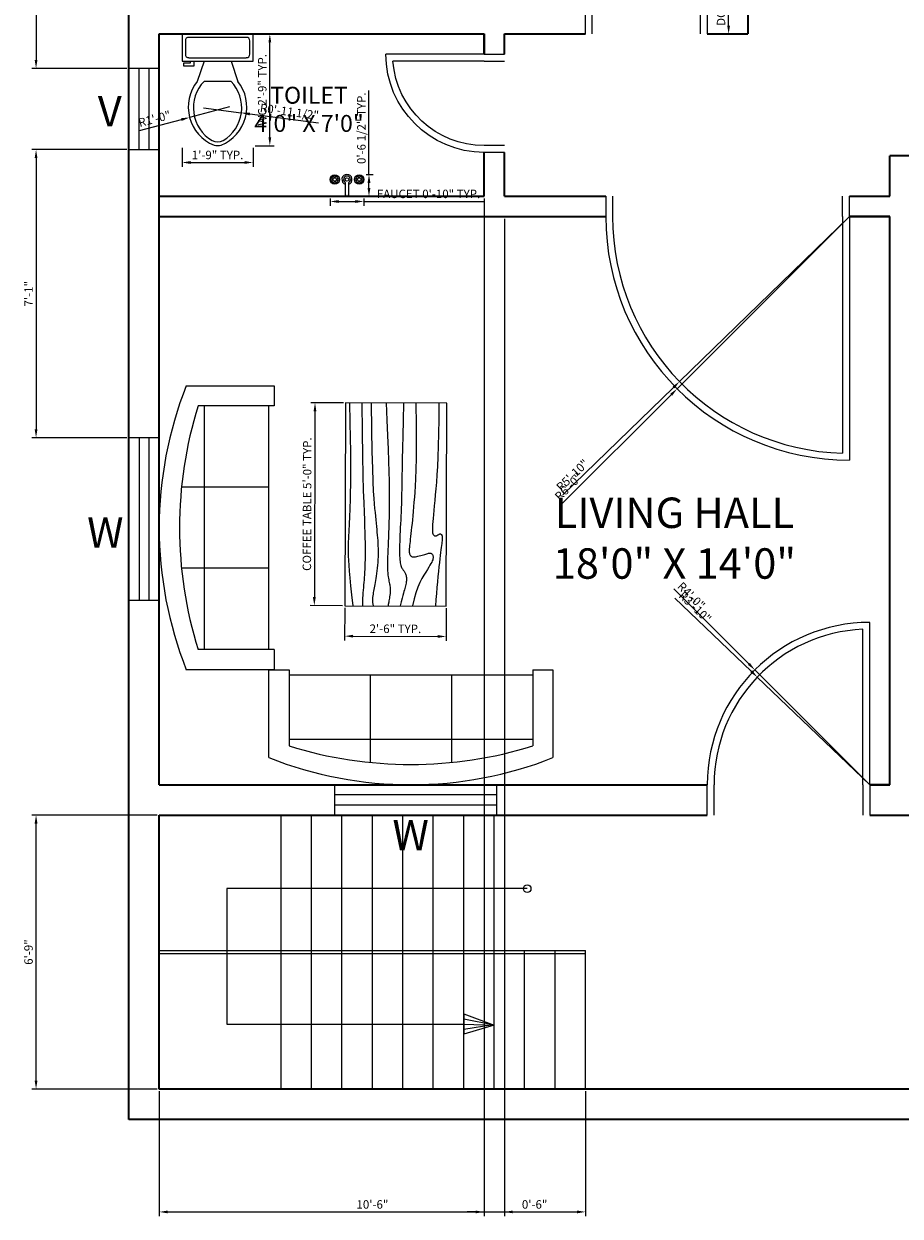
# Model space of a CAD drawing. Units: inches. Extents: x 1025 to 3479, y 1594 to 2212.
# Tile 4 of 9: x 2313 to 2572, y 1594 to 1947. Entities that reach past the tile are written whole.
import ezdxf

# ---------------------------------------------------------------- set-up
doc = ezdxf.new("R2010")
doc.units = ezdxf.units.IN
for name, color, linetype, lineweight in [('A-ANNO-DIMS', 1, 'Continuous', 18), ('A-ANNO-SYMB', 1, 'Continuous', 13), ('A-ANNO-TEXT', 7, 'Continuous', 18), ('A-AREA-IDEN', 4, 'Continuous', 18), ('A-DOOR', 4, 'Continuous', 18), ('A-FLOR-FIXT', 9, 'Continuous', 18), ('A-FLOR-STRS', 7, 'Continuous', 18), ('A-FURN', 8, 'Continuous', 13), ('A-GLAZ', 3, 'Continuous', 18), ('A-WALL', 7, 'Continuous', 35)]:
    doc.layers.add(name, color=color, linetype=linetype, lineweight=lineweight)
doc.styles.get("Standard").update_dxf_attribs({"font": 'arial.ttf'})
doc.dimstyles.new('ISO-25', dxfattribs={"dimtxt": 2.5, "dimasz": 2.5, "dimexe": 1.25, "dimexo": 0.625, "dimtad": 1, "dimdec": 0, "dimlunit": 3, "dimtxsty": 'Standard', "dimcen": 2.5, "dimadec": 0, "dimazin": 0, "dimtfac": 1, "dimtdec": 0, "dimtmove": 0, "dimatfit": 3, "dimfxl": 1, "dimarcsym": 0})

# ---------------------------------------------------------------- blocks, each defined once
blk = doc.blocks.new('Toilet - top')
for p, q in [((9.5, -6), (9.5, -2)), ((-10, -8.5), (-8, -8.5)), ((-10, -9.5), (-10, -8.5)), ((-7, -9.5), (-10, -9.5)), ((-8, -8.5), (-8, -8)), ((-7, -8), (-7, -9.5)), ((-4, -8), (-6, -14)), ((4, -8), (6, -14)), ((4, -14), (-4, -14))]:
    blk.add_line(p, q)
blk.add_lwpolyline([(10.5, -8), (10.5, 0), (-10.5, 0), (-10.5, -8)], close=True)
for points in [[(-9.5, -2), (-9.5, -6)], [(8.5, -1), (-8.5, -1)], [(-8.5, -7), (8.5, -7)]]:
    blk.add_lwpolyline(points)
for centre, radius, start, end in [((-8.62, -1.88), 0.884, 81.8699, 188.1301), ((8.62, -1.88), 0.884, 351.8699, 98.1301), ((-8.62, -6.12), 0.884, 171.8699, 278.1301), ((8.62, -6.12), 0.884, 261.8699, 8.1301), ((3.52, -21.58), 12.17, 141.4691, 247.9714), ((4.2, -21.82), 11.33, 136.3677, 238.9468), ((-3.52, -21.58), 12.17, 292.0284, 38.5307), ((-4.2, -21.82), 11.33, 301.053, 43.6321), ((0, -27.88), 4, 245.7318, 294.2682), ((0, -29), 4, 254.8605, 285.1395)]:
    blk.add_arc(centre, radius, start, end)
blk = doc.blocks.new('Faucet - Bathroom top')
for p, q in [((-4.107, 0.125), (-4.375, 0.125)), ((-3.75, 0.4788), (-3.75, 0.75)), ((-3.5, 0.482), (-3.5, 0.75)), ((-3.1461, 0.125), (-2.875, 0.125)), ((3.143, 0.125), (2.875, 0.125)), ((3.5, 0.4788), (3.5, 0.75)), ((3.75, 0.482), (3.75, 0.75)), ((4.1039, 0.125), (4.375, 0.125)), ((-4.1039, -0.125), (-4.375, -0.125)), ((-3.75, -0.4821), (-3.75, -0.75)), ((-3.5, -0.4789), (-3.5, -0.75)), ((-3.143, -0.125), (-2.875, -0.125)), ((-0.5, -0.8639), (-0.5, -4.5)), ((0.5, -4.5), (0.5, -0.8631)), ((3.1461, -0.125), (2.875, -0.125)), ((3.5, -0.4821), (3.5, -0.75)), ((3.75, -0.4789), (3.75, -0.75)), ((4.107, -0.125), (4.375, -0.125))]:
    blk.add_line(p, q)
for centre, radius in [((-3.625, 0), 1.375), ((-4.625, 0), 0.2795), ((-3.625, 0), 0.5), ((-3.625, 1), 0.2795), ((-2.625, 0), 0.2795), ((0, 0), 0.5), ((3.625, 0), 1.375), ((2.625, 0), 0.2795), ((3.625, 0), 0.5), ((3.625, 1), 0.2795), ((4.625, 0), 0.2795), ((-3.625, -1), 0.2795), ((3.625, -1), 0.2795)]:
    blk.add_circle(centre, radius)
for centre, radius, start, end in [((-3.625, 0), 1, 105.2407, 164.2093), ((-3.625, 0), 1, 16.44125, 74.07887), ((0, 0), 1.5, 289.6514, 250.3603), ((0, 0), 1, 300.3431, 239.7554), ((3.625, 0), 1, 106.12, 164.0884), ((3.625, 0), 1, 16.23422, 73.90469), ((-3.625, 0), 1, 196.2342, 253.9047), ((-3.625, 0), 1, 286.12, 344.0884), ((3.625, 0), 1, 196.4413, 254.0789), ((3.625, 0), 1, 285.2407, 344.2093), ((0, -4.5), 0.5, 180, 0)]:
    blk.add_arc(centre, radius, start, end)
blk = doc.blocks.new('Sofa - Roundback 7 ft.')
for p, q in [((-12.00002, -32.4421), (-12.00003, -6.5971)), ((11.99997, -32.4421), (11.99998, -6.5971)), ((-36.000027, -34), (-36.000027, -11.4696)), ((-35.999844, -13.3819), (35.9998, -13.3819)), ((35.99998, -34), (35.99998, -11.4696)), ((-36.000027, -32.4421), (35.99998, -32.4421))]:
    blk.add_line(p, q)
for points in [[(-36.000027, -34), (-42.000027, -34), (-42.000027, -8)], [(41.99998, -8), (41.99998, -34), (35.99998, -34)]]:
    blk.add_lwpolyline(points)
for centre, radius, start, end in [((0, -114.25), 114.25, 68.43141, 111.5686), ((-0.00001, -127.1968), 121.1968, 72.72033, 107.2797)]:
    blk.add_arc(centre, radius, start, end)
blk = doc.blocks.new('Table - Rectangular Woodgrain 60 x 30 in.')
for p, q in [((0, 0), (0, -30)), ((60, 0), (0, 0)), ((60, -30), (60, 0)), ((0, -30), (60, -30))]:
    blk.add_line(p, q)
for points in [[(0, -2.4), (4.8155, -2.418), (9.0302, -2.4688), (12.709, -2.5477), (15.9167, -2.65), (18.7181, -2.7711), (21.1781, -2.9063), (23.3616, -3.0508), (25.3333, -3.2), (27.1477, -3.3495), (28.8172, -3.4958), (30.3437, -3.636), (31.7291, -3.7667), (32.9756, -3.8849), (34.0849, -3.9875), (35.059, -4.0714), (35.9, -4.1334), (36.6114, -4.1711), (37.2041, -4.1854), (37.6906, -4.1779), (38.0833, -4.15), (38.3948, -4.1034), (38.6375, -4.0396), (38.8239, -3.9602), (38.9666, -3.8667), (39.0764, -3.7608), (39.1573, -3.6448), (39.2116, -3.521), (39.2416, -3.3917), (39.2498, -3.2593), (39.2385, -3.1261), (39.21, -2.9944), (39.1666, -2.8667), (39.111, -2.7447), (39.0468, -2.6281), (38.978, -2.5163), (38.9083, -2.4083), (38.8418, -2.3035), (38.7823, -2.201), (38.7337, -2.1001), (38.7, -2), (38.6844, -1.9003), (38.6875, -1.8021), (38.7094, -1.707), (38.75, -1.6167), (38.8094, -1.5326), (38.8875, -1.4563), (38.9844, -1.3893), (39.1, -1.3333), (39.2351, -1.2896), (39.3937, -1.2583), (39.5804, -1.2396), (39.8, -1.2333), (40.057, -1.2396), (40.3562, -1.2583), (40.7023, -1.2896), (41.1, -1.3333), (41.5547, -1.3895), (42.0755, -1.4573), (42.6721, -1.5361), (43.3542, -1.625), (44.1316, -1.7233), (45.014, -1.8302), (46.0114, -1.9449), (47.1333, -2.0667), (48.3862, -2.1947), (49.7625, -2.3281), (51.2513, -2.4663), (52.8416, -2.6083), (54.5226, -2.7535), (56.2833, -2.9011), (58.1127, -3.0501), (60, -3.2)], [(0, -9.2), (6.5759, -9.0858), (11.9385, -9.0365), (16.2527, -9.0418), (19.6833, -9.0917), (22.3952, -9.1759), (24.5531, -9.2844), (26.322, -9.4069), (27.8666, -9.5333), (29.3241, -9.6553), (30.7203, -9.7719), (32.0532, -9.8837), (33.3208, -9.9917), (34.5213, -10.0965), (35.6526, -10.199), (36.7128, -10.2999), (37.7, -10.4), (38.6129, -10.4996), (39.4531, -10.5969), (40.223, -10.6895), (40.925, -10.775), (41.5613, -10.8512), (42.1344, -10.9156), (42.6465, -10.966), (43.1, -11), (43.4976, -11.0158), (43.8437, -11.0136), (44.143, -10.9942), (44.4, -10.9583), (44.6195, -10.9069), (44.8062, -10.8406), (44.9648, -10.7603), (45.1, -10.6667), (45.2155, -10.5598), (45.3114, -10.4365), (45.3871, -10.2929), (45.4416, -10.125), (45.4743, -9.929), (45.4844, -9.7011), (45.4709, -9.4371), (45.4333, -9.1333), (45.3716, -8.7883), (45.2896, -8.4104), (45.1919, -8.0107), (45.0833, -7.6), (44.9685, -7.1893), (44.8521, -6.7896), (44.7388, -6.4117), (44.6333, -6.0667), (44.54, -5.7628), (44.4614, -5.4979), (44.4001, -5.2675), (44.3583, -5.0667), (44.3384, -4.8909), (44.3427, -4.7354), (44.3736, -4.5956), (44.4333, -4.4667), (44.5236, -4.3453), (44.6427, -4.2333), (44.7884, -4.1339), (44.9583, -4.05), (45.1501, -3.9849), (45.3614, -3.9417), (45.59, -3.9234), (45.8333, -3.9333), (46.0915, -3.9749), (46.3734, -4.0531), (46.6906, -4.1736), (47.0542, -4.3417), (47.4756, -4.5629), (47.9661, -4.8427), (48.5372, -5.1866), (49.2, -5.6), (49.9676, -6.0844), (50.8594, -6.625), (51.8965, -7.2031), (53.1, -7.8), (54.491, -8.3969), (56.0906, -8.975), (57.9199, -9.5156), (60, -10)], [(0, -12.8), (5.1847, -12.9322), (9.6213, -13.0323), (13.3963, -13.1059), (16.5958, -13.1583), (19.3063, -13.1952), (21.614, -13.2219), (23.6054, -13.2439), (25.3666, -13.2667), (26.9728, -13.2947), (28.4531, -13.3281), (29.8256, -13.3663), (31.1083, -13.4083), (32.3191, -13.4535), (33.476, -13.501), (34.597, -13.5501), (35.7, -13.6), (36.7984, -13.6497), (37.8875, -13.6979), (38.9578, -13.743), (40, -13.7833), (41.0047, -13.8174), (41.9625, -13.8438), (42.864, -13.8607), (43.7, -13.8667), (44.4631, -13.8604), (45.1552, -13.8417), (45.7801, -13.8104), (46.3416, -13.7667), (46.8439, -13.7104), (47.2906, -13.6417), (47.6858, -13.5604), (48.0333, -13.4667), (48.3375, -13.3608), (48.6042, -13.2448), (48.8396, -13.121), (49.05, -12.9917), (49.2417, -12.8593), (49.4208, -12.7261), (49.5937, -12.5944), (49.7667, -12.4667), (49.9452, -12.3451), (50.1323, -12.2313), (50.3303, -12.1268), (50.5416, -12.0333), (50.7686, -11.9524), (51.0135, -11.8854), (51.2788, -11.8341), (51.5666, -11.8), (51.8785, -11.7843), (52.2116, -11.7865), (52.562, -11.8059), (52.926, -11.8417), (53.2998, -11.8931), (53.6795, -11.9594), (54.0614, -12.0397), (54.4416, -12.1333), (54.8223, -12.2401), (55.2293, -12.3625), (55.6942, -12.5037), (56.2489, -12.6667), (56.9251, -12.8547), (57.7545, -13.0708), (58.7689, -13.3182), (60, -13.6)], [(0, -18), (5.124, -17.7273), (9.6609, -17.5057), (13.6705, -17.3303), (17.2125, -17.1958), (20.3467, -17.0973), (23.1328, -17.0297), (25.6307, -16.9878), (27.9, -16.9667), (29.9928, -16.9617), (31.9302, -16.9703), (33.7254, -16.9907), (35.3917, -17.0208), (36.9423, -17.0588), (38.3906, -17.1026), (39.7499, -17.1503), (41.0333, -17.2), (42.2519, -17.2496), (43.4073, -17.2969), (44.4986, -17.3395), (45.525, -17.375), (46.4858, -17.4012), (47.3802, -17.4156), (48.2074, -17.416), (48.9667, -17.4), (49.6583, -17.3662), (50.2872, -17.3167), (50.8595, -17.2547), (51.3812, -17.1833), (51.8584, -17.1057), (52.2971, -17.025), (52.7034, -16.9443), (53.0833, -16.8667), (53.443, -16.7951), (53.789, -16.7313), (54.128, -16.6768), (54.4666, -16.6334), (54.8115, -16.6024), (55.1693, -16.5854), (55.5465, -16.5841), (55.95, -16.6), (56.3828, -16.6337), (56.8346, -16.6823), (57.2915, -16.7418), (57.7396, -16.8084), (58.165, -16.878), (58.5539, -16.9469), (58.8924, -17.0111), (59.1666, -17.0667), (59.3679, -17.1107), (59.5078, -17.1438), (59.6032, -17.1675), (59.6708, -17.1833), (59.7275, -17.193), (59.7901, -17.1979), (59.8753, -17.1998), (60, -17.2)], [(0, -22.4), (8.0098, -22.2501), (14.4094, -22.1011), (19.4168, -21.9535), (23.25, -21.8083), (26.1269, -21.6663), (28.2656, -21.5281), (29.884, -21.3947), (31.2, -21.2667), (32.3967, -21.1448), (33.5172, -21.0292), (34.5697, -20.9198), (35.5625, -20.8167), (36.5037, -20.7198), (37.4015, -20.6292), (38.2642, -20.5448), (39.1, -20.4667), (39.9164, -20.3951), (40.7187, -20.3313), (41.5117, -20.2768), (42.3, -20.2333), (43.0883, -20.2024), (43.8812, -20.1854), (44.6836, -20.1841), (45.5, -20.2), (46.3328, -20.234), (47.1747, -20.2844), (48.0163, -20.3488), (48.8479, -20.425), (49.66, -20.5106), (50.4429, -20.6031), (51.1872, -20.7004), (51.8833, -20.8), (52.5246, -20.8999), (53.1166, -20.9995), (53.6681, -21.0983), (54.1875, -21.1958), (54.6834, -21.2919), (55.1646, -21.3859), (55.6394, -21.4777), (56.1167, -21.5667), (56.6028, -21.6515), (57.0961, -21.7266), (57.5929, -21.7852), (58.0896, -21.8208), (58.5823, -21.8268), (59.0674, -21.7964), (59.5412, -21.723), (60, -21.6)], [(0, -25.2), (8.6355, -25.0504), (15.7026, -24.9031), (21.4049, -24.7606), (25.9458, -24.625), (29.529, -24.4988), (32.3578, -24.3844), (34.6359, -24.284), (36.5667, -24.2), (38.3213, -24.1341), (39.9417, -24.0854), (41.437, -24.0523), (42.8167, -24.0333), (44.0901, -24.0268), (45.2667, -24.0313), (46.3557, -24.0451), (47.3667, -24.0667), (48.309, -24.0947), (49.1928, -24.1287), (50.0284, -24.168), (50.826, -24.2125), (51.5959, -24.2617), (52.3483, -24.3151), (53.0935, -24.3725), (53.8417, -24.4334), (54.6009, -24.497), (55.3699, -24.561), (56.1454, -24.6226), (56.9239, -24.6792), (57.7021, -24.7279), (58.4764, -24.7662), (59.2435, -24.7911), (60, -24.8)], [(0, -28.8), (5.6867, -28.6681), (10.45, -28.5698), (14.407, -28.5012), (17.675, -28.4584), (20.3711, -28.4374), (22.6125, -28.4344), (24.5164, -28.4455), (26.2, -28.4667), (27.762, -28.4947), (29.2276, -28.5281), (30.6033, -28.5663), (31.8958, -28.6084), (33.1118, -28.6535), (34.2578, -28.7011), (35.3405, -28.7501), (36.3666, -28.8), (37.3443, -28.8497), (38.288, -28.8974), (39.2137, -28.9412), (40.1375, -28.9792), (41.0753, -29.0093), (42.0432, -29.0297), (43.0572, -29.0384), (44.1333, -29.0333), (45.2936, -29.0114), (46.5843, -28.9641), (48.0579, -28.8816), (49.7666, -28.7542), (51.7629, -28.5721), (54.0989, -28.3255), (56.8272, -28.0048), (60, -27.6)]]:
    blk.add_lwpolyline(points)
blk = doc.blocks.new('WIN-48IN')
for p, q in [((0, 48), (0, 0)), ((9, 48), (0, 48)), ((3, 48), (3, 0)), ((6, 0), (6, 48)), ((9, 0), (9, 48)), ((0, 0), (9, 0))]:
    blk.add_line(p, q)
blk = doc.blocks.new('VENT-24IN')
for p, q in [((24, 9), (0, 9)), ((0, 9), (0, 0)), ((24, 0), (24, 9)), ((24, 6), (0, 6)), ((0, 3), (24, 3)), ((0, 0), (24, 0))]:
    blk.add_line(p, q)
blk = doc.blocks.new('DOOR-SWING-36IN')
for p, q in [((0, 36), (6, 36)), ((0, 34), (6, 34)), ((0, 2), (6, 2)), ((6, 0), (0, 0)), ((6, 2), (39.94, 2)), ((6, 0), (42, 0))]:
    blk.add_line(p, q)
for radius, start in [(36, 0), (34, 3.3723)]:
    blk.add_arc((6, 0), radius, start, 90)
blk = doc.blocks.new('DOOR-SWING-29IN')
for p, q in [((0, 6), (0, 35)), ((2, 6), (2, 32.93)), ((0, 6), (0, 0)), ((2, 6), (2, 0)), ((27, 0), (27, 6)), ((29, 0), (29, 6))]:
    blk.add_line(p, q)
for radius, end in [(29, 90), (27, 85.752)]:
    blk.add_arc((0, 6), radius, 0, end)
blk = doc.blocks.new('*D28')
at = {"layer": 'A-ANNO-DIMS', "color": 0, "lineweight": -2, "transparency": 16777216}
for p, q in [((2381.17, 1943.86), (2386.75, 1943.86)), ((2385.5, 1913.32), (2385.5, 1941.36)), ((2381.17, 1910.82), (2386.75, 1910.82))]:
    blk.add_line(p, q, dxfattribs=at)
at = {"layer": 'A-ANNO-DIMS', "color": 0, "transparency": 16777216}
for points in [[(2385.09, 1941.36), (2385.92, 1941.36), (2385.5, 1943.86)], [(2385.09, 1913.32), (2385.92, 1913.32), (2385.5, 1910.82)]]:
    blk.add_solid(points, dxfattribs=at)
at = {"layer": 'Defpoints', "color": 0, "transparency": 16777216}
for p in [(2380.55, 1943.86), (2385.5, 1943.86), (2380.55, 1910.82)]:
    blk.add_point(p, dxfattribs=at)
at = {"layer": 'A-ANNO-DIMS', "color": 0, "transparency": 16777216, "insert": (2383.59, 1927.34), "char_height": 2.5, "attachment_point": 5, "rotation": 90}
blk.add_mtext('WC 2\'-9" TYP.', dxfattribs=at)
blk = doc.blocks.new('*D29')
at = {"layer": 'A-ANNO-DIMS', "color": 0, "lineweight": -2, "transparency": 16777216}
for p, q in [((2359.55, 1910.19), (2359.55, 1904.61)), ((2380.55, 1910.19), (2380.55, 1904.61)), ((2362.05, 1905.86), (2378.05, 1905.86))]:
    blk.add_line(p, q, dxfattribs=at)
at = {"layer": 'A-ANNO-DIMS', "color": 0, "transparency": 16777216}
for points in [[(2362.05, 1906.28), (2362.05, 1905.44), (2359.55, 1905.86)], [(2378.05, 1906.28), (2378.05, 1905.44), (2380.55, 1905.86)]]:
    blk.add_solid(points, dxfattribs=at)
at = {"layer": 'Defpoints', "color": 0, "transparency": 16777216}
for p in [(2359.55, 1910.82), (2380.55, 1910.82), (2380.55, 1905.86)]:
    blk.add_point(p, dxfattribs=at)
at = {"layer": 'A-ANNO-DIMS', "color": 0, "transparency": 16777216, "insert": (2370.05, 1907.76), "char_height": 2.5, "attachment_point": 5}
blk.add_mtext('1\'-9" TYP.', dxfattribs=at)
blk = doc.blocks.new('*D30')
at = {"layer": 'A-ANNO-DIMS', "color": 0, "lineweight": -2, "transparency": 16777216}
for p, q in [((2403.31, 1895.2), (2403.31, 1893.08)), ((2405.81, 1894.33), (2410.81, 1894.33)), ((2413.31, 1895.2), (2413.31, 1893.08)), ((2413.31, 1894.33), (2449.04, 1894.33))]:
    blk.add_line(p, q, dxfattribs=at)
at = {"layer": 'A-ANNO-DIMS', "color": 0, "transparency": 16777216}
for points in [[(2405.81, 1894.75), (2405.81, 1893.91), (2403.31, 1894.33)], [(2410.81, 1894.75), (2410.81, 1893.91), (2413.31, 1894.33)]]:
    blk.add_solid(points, dxfattribs=at)
at = {"layer": 'Defpoints', "color": 0, "transparency": 16777216}
for p in [(2403.31, 1895.83), (2413.31, 1895.83), (2413.31, 1894.33)]:
    blk.add_point(p, dxfattribs=at)
at = {"layer": 'A-ANNO-DIMS', "color": 0, "transparency": 16777216, "insert": (2432.42, 1896.25), "char_height": 2.5, "attachment_point": 5}
blk.add_mtext('FAUCET 0\'-10" TYP.', dxfattribs=at)
blk = doc.blocks.new('*D31')
at = {"layer": 'A-ANNO-DIMS', "color": 0, "lineweight": -2, "transparency": 16777216}
for p, q in [((2414.81, 1902.33), (2414.81, 1927.14)), ((2413.93, 1902.33), (2416.06, 1902.33)), ((2414.81, 1898.33), (2414.81, 1899.83)), ((2413.93, 1895.83), (2416.06, 1895.83))]:
    blk.add_line(p, q, dxfattribs=at)
at = {"layer": 'A-ANNO-DIMS', "color": 0, "transparency": 16777216}
for points in [[(2414.39, 1899.83), (2415.23, 1899.83), (2414.81, 1902.33)], [(2414.39, 1898.33), (2415.23, 1898.33), (2414.81, 1895.83)]]:
    blk.add_solid(points, dxfattribs=at)
at = {"layer": 'Defpoints', "color": 0, "transparency": 16777216}
for p in [(2413.31, 1902.33), (2414.81, 1902.33), (2413.31, 1895.83)]:
    blk.add_point(p, dxfattribs=at)
at = {"layer": 'A-ANNO-DIMS', "color": 0, "transparency": 16777216, "insert": (2412.89, 1915.99), "char_height": 2.5, "attachment_point": 5, "rotation": 90}
blk.add_mtext('0\'-6 1/2" TYP.', dxfattribs=at)
blk = doc.blocks.new('*D32')
at = {"layer": 'A-ANNO-DIMS', "color": 0, "lineweight": -2, "transparency": 16777216}
for p, q in [((2515.45, 1985.86), (2522.37, 1985.86)), ((2521.12, 1946.36), (2521.12, 1983.36)), ((2515.45, 1943.86), (2522.37, 1943.86))]:
    blk.add_line(p, q, dxfattribs=at)
at = {"layer": 'A-ANNO-DIMS', "color": 0, "transparency": 16777216}
for points in [[(2520.71, 1983.36), (2521.54, 1983.36), (2521.12, 1985.86)], [(2520.71, 1946.36), (2521.54, 1946.36), (2521.12, 1943.86)]]:
    blk.add_solid(points, dxfattribs=at)
at = {"layer": 'Defpoints', "color": 0, "transparency": 16777216}
for p in [(2514.82, 1985.86), (2521.12, 1985.86), (2514.82, 1943.86)]:
    blk.add_point(p, dxfattribs=at)
at = {"layer": 'A-ANNO-DIMS', "color": 0, "transparency": 16777216, "insert": (2519.2, 1964.86), "char_height": 2.5, "attachment_point": 5, "rotation": 90}
blk.add_mtext('DOOR SWING 3\'-6" TYP.', dxfattribs=at)
blk = doc.blocks.new('*D38')
at = {"layer": 'A-ANNO-DIMS', "color": 0, "lineweight": -2, "transparency": 16777216}
for p, q in [((2407.23, 1834.79), (2397.6, 1834.82)), ((2398.84, 1832.32), (2398.66, 1777.32)), ((2407.02, 1774.79), (2397.4, 1774.82))]:
    blk.add_line(p, q, dxfattribs=at)
at = {"layer": 'A-ANNO-DIMS', "color": 0, "transparency": 16777216}
for points in [[(2398.43, 1832.32), (2399.26, 1832.32), (2398.85, 1834.82)], [(2398.24, 1777.32), (2399.07, 1777.32), (2398.65, 1774.82)]]:
    blk.add_solid(points, dxfattribs=at)
at = {"layer": 'Defpoints', "color": 0, "transparency": 16777216}
for p in [(2407.85, 1834.79), (2398.65, 1774.82), (2407.65, 1774.79)]:
    blk.add_point(p, dxfattribs=at)
at = {"layer": 'A-ANNO-DIMS', "color": 0, "transparency": 16777216, "insert": (2396.83, 1804.83), "char_height": 2.5, "attachment_point": 5, "rotation": 89.8036}
blk.add_mtext('COFFEE TABLE 5\'-0" TYP.', dxfattribs=at)
blk = doc.blocks.new('*D39')
at = {"layer": 'A-ANNO-DIMS', "color": 0, "lineweight": -2, "transparency": 16777216}
for p, q in [((2407.64, 1774.16), (2407.61, 1764.54)), ((2437.64, 1774.06), (2437.61, 1764.44)), ((2410.12, 1765.78), (2435.12, 1765.69))]:
    blk.add_line(p, q, dxfattribs=at)
at = {"layer": 'A-ANNO-DIMS', "color": 0, "transparency": 16777216}
for points in [[(2410.12, 1766.2), (2410.11, 1765.36), (2407.62, 1765.79)], [(2435.12, 1766.11), (2435.11, 1765.28), (2437.62, 1765.69)]]:
    blk.add_solid(points, dxfattribs=at)
at = {"layer": 'Defpoints', "color": 0, "transparency": 16777216}
for p in [(2407.65, 1774.79), (2437.65, 1774.69), (2437.62, 1765.69)]:
    blk.add_point(p, dxfattribs=at)
at = {"layer": 'A-ANNO-DIMS', "color": 0, "transparency": 16777216, "insert": (2422.62, 1767.64), "char_height": 2.5, "attachment_point": 5, "rotation": 359.8036}
blk.add_mtext('2\'-6" TYP.', dxfattribs=at)
blk = doc.blocks.new('*D59')
at = {"layer": 'A-ANNO-DIMS', "color": 0, "lineweight": -2, "transparency": 16777216}
for p, q in [((2343.12, 2008.89), (2315.14, 2008.89)), ((2316.39, 2006.39), (2316.39, 1936.18)), ((2343.2, 1933.68), (2315.14, 1933.68))]:
    blk.add_line(p, q, dxfattribs=at)
at = {"layer": 'A-ANNO-DIMS', "color": 0, "transparency": 16777216}
for points in [[(2315.98, 2006.39), (2316.81, 2006.39), (2316.39, 2008.89)], [(2315.98, 1936.18), (2316.81, 1936.18), (2316.39, 1933.68)]]:
    blk.add_solid(points, dxfattribs=at)
at = {"layer": 'Defpoints', "color": 0, "transparency": 16777216}
for p in [(2343.74, 2008.89), (2316.39, 1933.68), (2343.82, 1933.68)]:
    blk.add_point(p, dxfattribs=at)
at = {"layer": 'A-ANNO-DIMS', "color": 0, "transparency": 16777216, "insert": (2314.49, 1971.28), "char_height": 2.5, "attachment_point": 5, "rotation": 90}
blk.add_mtext('6\'-3"', dxfattribs=at)
blk = doc.blocks.new('*D60')
at = {"layer": 'A-ANNO-DIMS', "color": 0, "lineweight": -2, "transparency": 16777216}
for p, q in [((2343.2, 1909.68), (2315.14, 1909.68)), ((2316.39, 1907.18), (2316.39, 1826.95)), ((2343.22, 1824.45), (2315.14, 1824.45))]:
    blk.add_line(p, q, dxfattribs=at)
at = {"layer": 'A-ANNO-DIMS', "color": 0, "transparency": 16777216}
for points in [[(2315.98, 1907.18), (2316.81, 1907.18), (2316.39, 1909.68)], [(2315.98, 1826.95), (2316.81, 1826.95), (2316.39, 1824.45)]]:
    blk.add_solid(points, dxfattribs=at)
at = {"layer": 'Defpoints', "color": 0, "transparency": 16777216}
for p in [(2343.82, 1909.68), (2316.39, 1824.45), (2343.84, 1824.45)]:
    blk.add_point(p, dxfattribs=at)
at = {"layer": 'A-ANNO-DIMS', "color": 0, "transparency": 16777216, "insert": (2314.51, 1867.06), "char_height": 2.5, "attachment_point": 5, "rotation": 90}
blk.add_mtext('7\'-1"', dxfattribs=at)
blk = doc.blocks.new('*D68')
at = {"layer": 'A-ANNO-DIMS', "color": 0, "lineweight": -2, "transparency": 16777216}
for p, q in [((2448.82, 1895.24), (2448.82, 1594.26)), ((2454.82, 1889.24), (2454.82, 1594.26)), ((2446.32, 1595.51), (2443.82, 1595.51)), ((2448.82, 1595.51), (2454.82, 1595.51)), ((2457.32, 1595.51), (2467.72, 1595.51))]:
    blk.add_line(p, q, dxfattribs=at)
at = {"layer": 'A-ANNO-DIMS', "color": 0, "transparency": 16777216}
for points in [[(2446.32, 1595.93), (2446.32, 1595.1), (2448.82, 1595.51)], [(2457.32, 1595.93), (2457.32, 1595.1), (2454.82, 1595.51)]]:
    blk.add_solid(points, dxfattribs=at)
at = {"layer": 'Defpoints', "color": 0, "transparency": 16777216}
for p in [(2448.82, 1895.86), (2454.82, 1889.86), (2454.82, 1595.51)]:
    blk.add_point(p, dxfattribs=at)
at = {"layer": 'A-ANNO-DIMS', "color": 0, "transparency": 16777216, "insert": (2463.77, 1597.41), "char_height": 2.5, "attachment_point": 5}
blk.add_mtext('0\'-6"', dxfattribs=at)
blk = doc.blocks.new('*D80')
at = {"layer": 'A-ANNO-DIMS', "color": 0, "lineweight": -2, "transparency": 16777216}
for p, q in [((2352.82, 1631.24), (2352.82, 1594.26)), ((2478.82, 1631.24), (2478.82, 1594.26)), ((2355.32, 1595.51), (2476.32, 1595.51))]:
    blk.add_line(p, q, dxfattribs=at)
at = {"layer": 'A-ANNO-DIMS', "color": 0, "transparency": 16777216}
for points in [[(2355.32, 1595.93), (2355.32, 1595.1), (2352.82, 1595.51)], [(2476.32, 1595.93), (2476.32, 1595.1), (2478.82, 1595.51)]]:
    blk.add_solid(points, dxfattribs=at)
at = {"layer": 'Defpoints', "color": 0, "transparency": 16777216}
for p in [(2352.82, 1631.86), (2478.82, 1631.86), (2478.82, 1595.51)]:
    blk.add_point(p, dxfattribs=at)
at = {"layer": 'A-ANNO-DIMS', "color": 0, "transparency": 16777216, "insert": (2415.82, 1597.41), "char_height": 2.5, "attachment_point": 5}
blk.add_mtext('10\'-6"', dxfattribs=at)
blk = doc.blocks.new('*D81')
at = {"layer": 'A-ANNO-DIMS', "color": 0, "lineweight": -2, "transparency": 16777216}
for p, q in [((2352.2, 1712.86), (2315.14, 1712.86)), ((2316.39, 1634.36), (2316.39, 1710.36)), ((2352.2, 1631.86), (2315.14, 1631.86))]:
    blk.add_line(p, q, dxfattribs=at)
at = {"layer": 'A-ANNO-DIMS', "color": 0, "transparency": 16777216}
for points in [[(2315.98, 1710.36), (2316.81, 1710.36), (2316.39, 1712.86)], [(2315.98, 1634.36), (2316.81, 1634.36), (2316.39, 1631.86)]]:
    blk.add_solid(points, dxfattribs=at)
at = {"layer": 'Defpoints', "color": 0, "transparency": 16777216}
for p in [(2316.39, 1712.86), (2352.82, 1712.86), (2352.82, 1631.86)]:
    blk.add_point(p, dxfattribs=at)
at = {"layer": 'A-ANNO-DIMS', "color": 0, "transparency": 16777216, "insert": (2314.49, 1672.36), "char_height": 2.5, "attachment_point": 5, "rotation": 90}
blk.add_mtext('6\'-9"', dxfattribs=at)
blk = doc.blocks.new('*D86')
at = {"layer": 'A-ANNO-DIMS', "color": 0, "lineweight": -2, "transparency": 16777216}
for p, q in [((2556.82, 1889.86), (2505.91, 1838.95)), ((2471.73, 1804.77), (2504.14, 1837.18))]:
    blk.add_line(p, q, dxfattribs=at)
at = {"layer": 'A-ANNO-DIMS', "color": 0, "transparency": 16777216}
blk.add_solid([(2503.85, 1837.48), (2504.44, 1836.89), (2505.91, 1838.95)], dxfattribs=at)
at = {"layer": 'Defpoints', "color": 0, "transparency": 16777216}
for p in [(2556.82, 1889.86), (2505.91, 1838.95)]:
    blk.add_point(p, dxfattribs=at)
at = {"layer": 'A-ANNO-DIMS', "color": 0, "transparency": 16777216, "insert": (2474.02, 1809.75), "char_height": 2.5, "attachment_point": 5, "rotation": 45.0001}
blk.add_mtext('R6\'-0"', dxfattribs=at)
blk = doc.blocks.new('*D87')
at = {"layer": 'A-ANNO-DIMS', "color": 0, "lineweight": -2, "transparency": 16777216}
for p, q in [((2504.88, 1779.81), (2527.11, 1757.57)), ((2562.82, 1721.86), (2528.88, 1755.8))]:
    blk.add_line(p, q, dxfattribs=at)
at = {"layer": 'A-ANNO-DIMS', "color": 0, "transparency": 16777216}
blk.add_solid([(2527.41, 1757.87), (2526.82, 1757.28), (2528.88, 1755.8)], dxfattribs=at)
at = {"layer": 'Defpoints', "color": 0, "transparency": 16777216}
for p in [(2528.88, 1755.8), (2562.82, 1721.86)]:
    blk.add_point(p, dxfattribs=at)
at = {"layer": 'A-ANNO-DIMS', "color": 0, "transparency": 16777216, "insert": (2509.86, 1777.51), "char_height": 2.5, "attachment_point": 5, "rotation": 314.9998}
blk.add_mtext('R4\'-0"', dxfattribs=at)
blk = doc.blocks.new('*D93')
at = {"layer": 'A-ANNO-DIMS', "color": 0, "lineweight": -2, "transparency": 16777216}
for p, q in [((2373.57, 1922.28), (2361.8, 1919.19)), ((2347.01, 1915.3), (2359.38, 1918.55))]:
    blk.add_line(p, q, dxfattribs=at)
at = {"layer": 'A-ANNO-DIMS', "color": 0, "transparency": 16777216}
blk.add_solid([(2359.27, 1918.96), (2359.48, 1918.15), (2361.8, 1919.19)], dxfattribs=at)
at = {"layer": 'Defpoints', "color": 0, "transparency": 16777216}
for p in [(2373.57, 1922.28), (2361.8, 1919.19)]:
    blk.add_point(p, dxfattribs=at)
at = {"layer": 'A-ANNO-DIMS', "color": 0, "transparency": 16777216, "insert": (2351.5, 1918.45), "char_height": 2.5, "attachment_point": 5, "rotation": 14.7214}
blk.add_mtext('R1\'-0"', dxfattribs=at)
blk = doc.blocks.new('*D94')
at = {"layer": 'A-ANNO-DIMS', "color": 0, "lineweight": -2, "transparency": 16777216}
for p, q in [((2365.85, 1922.04), (2377.07, 1920.54)), ((2399.93, 1917.46), (2379.55, 1920.2))]:
    blk.add_line(p, q, dxfattribs=at)
at = {"layer": 'A-ANNO-DIMS', "color": 0, "transparency": 16777216}
blk.add_solid([(2379.61, 1920.61), (2379.5, 1919.79), (2377.07, 1920.54)], dxfattribs=at)
at = {"layer": 'Defpoints', "color": 0, "transparency": 16777216}
for p in [(2365.85, 1922.04), (2377.07, 1920.54)]:
    blk.add_point(p, dxfattribs=at)
at = {"layer": 'A-ANNO-DIMS', "color": 0, "transparency": 16777216, "insert": (2391.23, 1920.57), "char_height": 2.5, "attachment_point": 5, "rotation": 352.3428}
blk.add_mtext('R0\'-11 1/2"', dxfattribs=at)
blk = doc.blocks.new('*D95')
at = {"layer": 'A-ANNO-DIMS', "color": 0, "lineweight": -2, "transparency": 16777216}
for p, q in [((2556.82, 1889.86), (2506.62, 1841.08)), ((2472.12, 1807.54), (2504.83, 1839.33))]:
    blk.add_line(p, q, dxfattribs=at)
at = {"layer": 'A-ANNO-DIMS', "color": 0, "transparency": 16777216}
blk.add_solid([(2504.54, 1839.63), (2505.12, 1839.04), (2506.62, 1841.08)], dxfattribs=at)
at = {"layer": 'Defpoints', "color": 0, "transparency": 16777216}
for p in [(2556.82, 1889.86), (2506.62, 1841.08)]:
    blk.add_point(p, dxfattribs=at)
at = {"layer": 'A-ANNO-DIMS', "color": 0, "transparency": 16777216, "insert": (2475.18, 1813.17), "char_height": 2.5, "attachment_point": 5, "rotation": 44.1812}
blk.add_mtext('R5\'-10"', dxfattribs=at)
blk = doc.blocks.new('*D96')
at = {"layer": 'A-ANNO-DIMS', "color": 0, "lineweight": -2, "transparency": 16777216}
for p, q in [((2505.24, 1776.99), (2527.79, 1755.4)), ((2562.82, 1721.86), (2529.6, 1753.67))]:
    blk.add_line(p, q, dxfattribs=at)
at = {"layer": 'A-ANNO-DIMS', "color": 0, "transparency": 16777216}
blk.add_solid([(2528.08, 1755.7), (2527.5, 1755.1), (2529.6, 1753.67)], dxfattribs=at)
at = {"layer": 'Defpoints', "color": 0, "transparency": 16777216}
for p in [(2529.6, 1753.67), (2562.82, 1721.86)]:
    blk.add_point(p, dxfattribs=at)
at = {"layer": 'A-ANNO-DIMS', "color": 0, "transparency": 16777216, "insert": (2510.98, 1774.14), "char_height": 2.5, "attachment_point": 5, "rotation": 316.2461}
blk.add_mtext('R3\'-10"', dxfattribs=at)

msp = doc.modelspace()

# ---------------------------------------------------------------- linework, layer by layer
at = {"layer": 'A-ANNO-SYMB'}
for p, q in [((2461.58, 1691.11), (2372.74, 1691.11)), ((2372.74, 1691.11), (2372.74, 1651.06)), ((2442.82, 1651.06), (2442.82, 1654.06)), ((2442.82, 1654.06), (2442.82, 1651.06)), ((2442.82, 1654.06), (2451.82, 1650.77)), ((2372.74, 1651.06), (2442.82, 1651.06)), ((2451.82, 1650.77), (2442.82, 1652.56)), ((2442.82, 1652.56), (2442.82, 1649.56)), ((2442.82, 1651.06), (2442.82, 1648.06)), ((2442.82, 1651.06), (2451.82, 1650.77)), ((2442.82, 1649.56), (2451.44, 1650.91)), ((2451.82, 1650.77), (2442.82, 1648.06)), ((2451.44, 1650.91), (2451.44, 1650.67))]:
    msp.add_line(p, q, dxfattribs=at)
msp.add_circle((2461.58, 1691.11), 1.12, dxfattribs=at)
at = {"layer": 'A-DOOR'}
for p, q in [((2419.89, 1935.86), (2419.82, 1935.86)), ((2484.82, 1895.86), (2484.82, 1889.86)), ((2486.82, 1895.86), (2486.82, 1889.86)), ((2554.82, 1889.86), (2554.82, 1895.86)), ((2556.82, 1889.86), (2556.82, 1895.86)), ((2554.82, 1889.86), (2554.82, 1819.89)), ((2556.82, 1889.86), (2556.82, 1817.86)), ((2554.82, 1817.89), (2554.82, 1817.86)), ((2560.82, 1769.82), (2560.82, 1769.86)), ((2560.82, 1721.86), (2560.82, 1767.82)), ((2562.82, 1721.86), (2562.82, 1769.86)), ((2514.82, 1712.86), (2514.82, 1721.86)), ((2516.82, 1712.86), (2516.82, 1721.86)), ((2560.82, 1721.86), (2560.82, 1712.86)), ((2562.82, 1721.86), (2562.82, 1712.86))]:
    msp.add_line(p, q, dxfattribs=at)
for centre, radius, start, end in [((2556.82, 1889.86), 72, 180, 270), ((2556.82, 1889.86), 70, 180, 268.3628), ((2562.82, 1721.86), 48, 90, 180), ((2562.82, 1721.86), 46, 92.4919, 180)]:
    msp.add_arc(centre, radius, start, end, dxfattribs=at)
at = {"layer": 'A-FLOR-STRS'}
for p, q in [((2388.82, 1631.86), (2388.82, 1712.86)), ((2397.82, 1631.86), (2397.82, 1712.86)), ((2406.82, 1631.86), (2406.82, 1712.86)), ((2415.82, 1631.86), (2415.82, 1712.86)), ((2424.82, 1631.86), (2424.82, 1712.86)), ((2433.82, 1631.86), (2433.82, 1712.86)), ((2442.82, 1631.86), (2442.82, 1712.86)), ((2451.82, 1631.86), (2451.82, 1712.86)), ((2352.82, 1672.86), (2454.82, 1672.86)), ((2478.82, 1671.86), (2352.82, 1671.86)), ((2454.82, 1672.86), (2478.82, 1672.86)), ((2460.82, 1631.86), (2460.82, 1672.86)), ((2469.82, 1631.86), (2469.82, 1672.86)), ((2478.82, 1631.86), (2478.82, 1672.86))]:
    msp.add_line(p, q, dxfattribs=at)
at = {"layer": 'A-WALL'}
for p, q in [((2343.82, 1622.86), (2343.82, 2102.86)), ((2526.82, 1967.86), (2526.82, 1943.86)), ((2352.82, 1943.86), (2448.82, 1943.86)), ((2352.82, 1721.86), (2352.82, 1943.86)), ((2448.82, 1943.86), (2448.82, 1937.86)), ((2448.82, 1937.86), (2448.82, 1943.86)), ((2454.82, 1943.86), (2478.82, 1943.86)), ((2454.82, 1937.86), (2454.82, 1943.86)), ((2514.82, 1943.86), (2520.82, 1943.86)), ((2520.82, 1943.86), (2526.82, 1943.86)), ((2448.82, 1895.86), (2448.82, 1908.86)), ((2454.82, 1895.86), (2454.82, 1908.86)), ((2568.82, 1895.86), (2568.82, 1907.86)), ((2574.82, 1907.86), (2568.82, 1907.86)), ((2352.82, 1895.86), (2448.82, 1895.86)), ((2454.82, 1895.86), (2484.82, 1895.86)), ((2556.82, 1895.86), (2568.82, 1895.86)), ((2352.82, 1889.86), (2454.82, 1889.86)), ((2454.82, 1889.86), (2484.82, 1889.86)), ((2568.82, 1889.86), (2556.82, 1889.86)), ((2556.82, 1889.86), (2568.82, 1889.86)), ((2568.82, 1721.86), (2568.82, 1889.86)), ((2352.82, 1721.86), (2454.82, 1721.86)), ((2454.82, 1721.86), (2514.82, 1721.86)), ((2568.82, 1721.86), (2562.82, 1721.86)), ((2562.82, 1721.86), (2568.82, 1721.86)), ((2352.82, 1631.86), (2352.82, 1712.86)), ((2352.82, 1712.86), (2454.82, 1712.86)), ((2454.82, 1712.86), (2514.82, 1712.86)), ((2562.82, 1712.86), (2568.82, 1712.86)), ((2568.82, 1712.86), (2577.82, 1712.86)), ((2694.82, 1631.86), (2352.82, 1631.86)), ((2703.82, 1622.86), (2343.82, 1622.86))]:
    msp.add_line(p, q, dxfattribs=at)

# ---------------------------------------------------------------- block references
at = {"layer": 'A-DOOR', "rotation": 89.99999999999888}
msp.add_blockref('DOOR-SWING-36IN', (2514.82, 1943.86), dxfattribs=at)
at = {"layer": 'A-DOOR', "extrusion": (0, 0, -1), "zscale": -1, "rotation": 270.0000000000007}
msp.add_blockref('DOOR-SWING-29IN', (-2454.82, 1937.86), dxfattribs=at)
at = {"layer": 'A-FLOR-FIXT'}
for name, p in [('Toilet - top', (2370.05, 1943.86)), ('Faucet - Bathroom top', (2408.31, 1900.83))]:
    msp.add_blockref(name, p, dxfattribs=at)
at = {"layer": 'A-FURN'}
for name, p, rotation in [('Sofa - Roundback 7 ft.', (2352.8, 1797.85), 90), ('Table - Rectangular Woodgrain 60 x 30 in.', (2437.85, 1834.69), 269.8036337053011), ('Sofa - Roundback 7 ft.', (2427.2, 1721.85), 180)]:
    msp.add_blockref(name, p, dxfattribs=dict(at, rotation=rotation))
at = {"layer": 'A-GLAZ'}
for name, p, rotation in [('VENT-24IN', (2343.82, 1933.68), 270.0000000000037), ('WIN-48IN', (2404.61, 1721.86), 270.0000000000005)]:
    msp.add_blockref(name, p, dxfattribs=dict(at, rotation=rotation))
msp.add_blockref('WIN-48IN', (2343.84, 1776.45), dxfattribs=at)

# ---------------------------------------------------------------- texts
at = {"layer": 'A-ANNO-TEXT', "char_height": 9, "attachment_point": 1}
for s, width, insert in [('\\pxqc;{V}', 7.8272, (2334.27, 1925.52)), ('\\pxqc;W', 15.8719, (2328.93, 1800.96)), ('\\pxqc;W', 15.8719, (2419.19, 1711.42))]:
    msp.add_mtext_dynamic_manual_height_columns(s, width=width, gutter_width=12.5, heights=[0], dxfattribs=dict(at, insert=insert))
at = {"layer": 'A-AREA-IDEN', "attachment_point": 1}
for s, width, insert, char_height in [('\\pxqc;TOILET \\P4\'0" X 7\'0" ', 51.1118, (2371.53, 1928.25), 5), ('\\pxqc;LIVING HALL \\P18\'0" X 14\'0"', 93.2353, (2458.48, 1806.77), 9)]:
    msp.add_mtext_dynamic_manual_height_columns(s, width=width, gutter_width=12.5, heights=[0], dxfattribs=dict(at, insert=insert, char_height=char_height))

# ---------------------------------------------------------------- dimensions: what is measured, and where the dimension line sits
at = {"layer": 'A-ANNO-DIMS'}
for base, p1, p2, picture, middle in [((2316.39, 1933.68), (2343.74, 2008.89), (2343.82, 1933.68), '*D59', (2314.49, 1971.28)), ((2316.39, 1824.45), (2343.82, 1909.68), (2343.84, 1824.45), '*D60', (2314.51, 1867.06)), ((2316.39, 1712.86), (2352.82, 1631.86), (2352.82, 1712.86), '*D81', (2314.49, 1672.36))]:
    dim = msp.add_linear_dim(base=base, p1=p1, p2=p2, angle=90, dimstyle='ISO-25', override={"dimdec": 1, "dimlfac": 1, "dimrnd": 0, "dimzin": 1, "dimdsep": 46, "dimlunit": 4, "dimfrac": 2}, dxfattribs=at)
    dim.commit()
    dim.dimension.update_dxf_attribs({"geometry": picture, "text_midpoint": middle})
for base, p1, p2, angle, text, picture, middle in [((2521.12, 1985.86), (2514.82, 1943.86), (2514.82, 1985.86), 90, 'DOOR SWING <> TYP.', '*D32', (2519.2, 1964.86)), ((2385.5, 1943.86), (2380.55, 1910.82), (2380.55, 1943.86), 90, 'WC <> TYP.', '*D28', (2383.59, 1927.34)), ((2414.81, 1902.33), (2413.31, 1895.83), (2413.31, 1902.33), 90, '<> TYP.', '*D31', (2412.89, 1915.99)), ((2398.65, 1774.82), (2407.85, 1834.79), (2407.65, 1774.79), 269.8036, 'COFFEE TABLE <> TYP.', '*D38', (2396.83, 1804.83)), ((2437.62, 1765.69), (2407.65, 1774.79), (2437.65, 1774.69), 359.8036, '<> TYP.', '*D39', (2422.62, 1767.64))]:
    dim = msp.add_linear_dim(base=base, p1=p1, p2=p2, angle=angle, text=text, dimstyle='ISO-25', override={"dimdec": 1, "dimlfac": 1, "dimrnd": 0, "dimzin": 1, "dimdsep": 46, "dimlunit": 4, "dimfrac": 2}, dxfattribs=at)
    dim.commit()
    dim.dimension.update_dxf_attribs({"geometry": picture, "text_midpoint": middle})
for center, mpoint, picture, middle in [((2373.57, 1922.28), (2361.8, 1919.19), '*D93', (2351.5, 1918.45)), ((2365.85, 1922.04), (2377.07, 1920.54), '*D94', (2391.23, 1920.57))]:
    dim = msp.add_radius_dim(center=center, mpoint=mpoint, dimstyle='ISO-25', override={"dimdec": 1, "dimlfac": 1, "dimrnd": 0, "dimzin": 1, "dimdsep": 46, "dimlunit": 4, "dimfrac": 2}, dxfattribs=at)
    dim.commit()
    dim.dimension.update_dxf_attribs({"geometry": picture, "text_midpoint": middle})
for base, p1, p2, text, picture, middle in [((2380.55, 1905.86), (2359.55, 1910.82), (2380.55, 1910.82), '<> TYP.', '*D29', (2370.05, 1907.76)), ((2413.31, 1894.33), (2403.31, 1895.83), (2413.31, 1895.83), 'FAUCET <> TYP.', '*D30', (2432.42, 1896.25))]:
    dim = msp.add_linear_dim(base=base, p1=p1, p2=p2, text=text, dimstyle='ISO-25', override={"dimdec": 1, "dimlfac": 1, "dimrnd": 0, "dimzin": 1, "dimdsep": 46, "dimlunit": 4, "dimfrac": 2}, dxfattribs=at)
    dim.commit()
    dim.dimension.update_dxf_attribs({"geometry": picture, "text_midpoint": middle})
for base, p1, p2, picture, middle in [((2454.82, 1595.51), (2448.82, 1895.86), (2454.82, 1889.86), '*D68', (2463.77, 1597.41)), ((2478.82, 1595.51), (2352.82, 1631.86), (2478.82, 1631.86), '*D80', (2415.82, 1597.41))]:
    dim = msp.add_linear_dim(base=base, p1=p1, p2=p2, dimstyle='ISO-25', override={"dimdec": 1, "dimlfac": 1, "dimrnd": 0, "dimzin": 1, "dimdsep": 46, "dimlunit": 4, "dimfrac": 2}, dxfattribs=at)
    dim.commit()
    dim.dimension.update_dxf_attribs({"geometry": picture, "text_midpoint": middle})
for center, mpoint, picture, middle in [((2556.82, 1889.86), (2505.91, 1838.95), '*D86', (2475.37, 1808.4)), ((2556.82, 1889.86), (2506.62, 1841.08), '*D95', (2476.5, 1811.81)), ((2562.82, 1721.86), (2528.88, 1755.8), '*D87', (2508.52, 1776.17)), ((2562.82, 1721.86), (2529.6, 1753.67), '*D96', (2509.66, 1772.76))]:
    dim = msp.add_radius_dim(center=center, mpoint=mpoint, dimstyle='ISO-25', override={"dimdec": 1, "dimlfac": 1, "dimrnd": 0, "dimzin": 1, "dimdsep": 46, "dimlunit": 4, "dimfrac": 2}, dxfattribs=at)
    dim.commit()
    dim.dimension.update_dxf_attribs({"geometry": picture, "text_midpoint": middle, "dimtype": 164})

doc.saveas('drawing.dxf')
